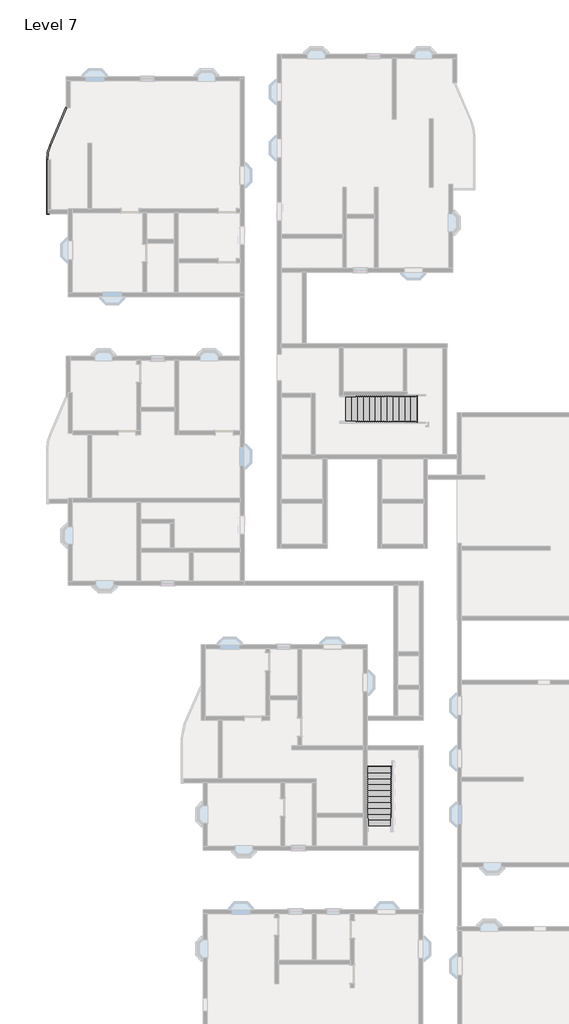
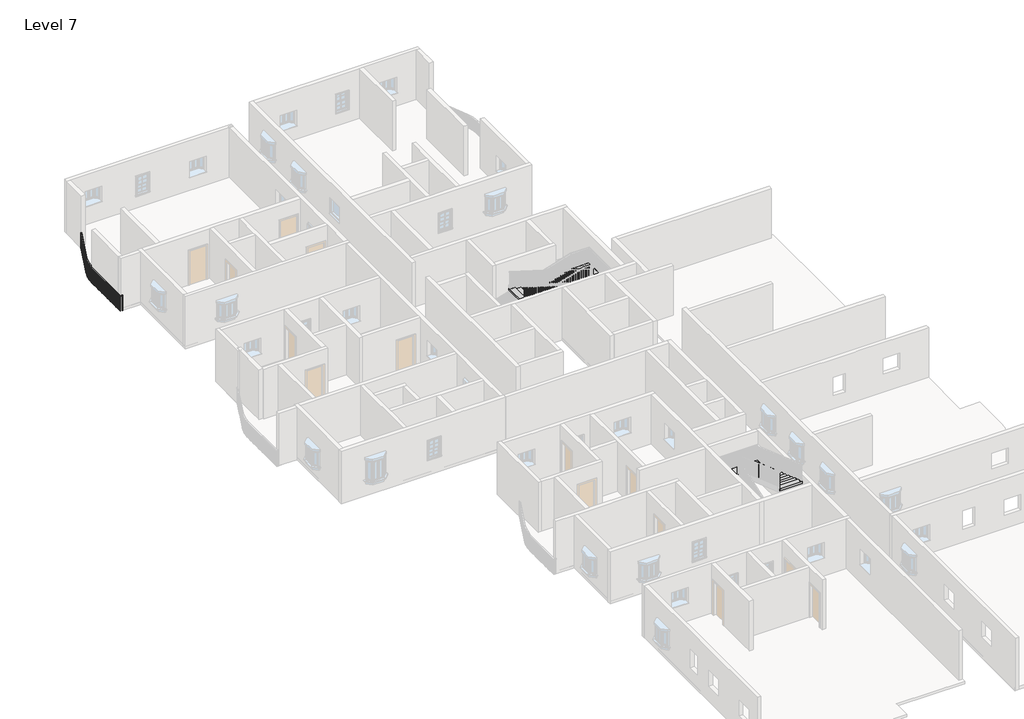
# One storey, part 12 of 14: 2 stair flights, 1 railing.
"""IFC4 building model written with IfcOpenShell, lengths in millimetres."""

from ifc_helpers import new_model, si_unit, frame, origin, place, context, project, spatial, polyline, circle_curve, outline, extrude, transform, mapped, element, save
from ifc_brep_helpers import plane_surface, cylinder_surface, revolved_surface, advanced_brep
from components import stair_flight_8b440c70, stair_flight_8f1750f9

model = new_model("IFC4")

# Units and contexts
model_context = context("Model", 3, world=origin())
ifc_project = project(units=[si_unit("LENGTHUNIT", "METRE", prefix="MILLI")], contexts=[model_context])

# Site, building, storey
site = spatial("IfcSite", under=ifc_project)
building = spatial("IfcBuilding", under=site)
storey = spatial("IfcBuildingStorey", under=building, Name="Level 7", Elevation=18288.0)

# Railing
placement = place(None, origin())
element("IfcRailing", 1, ObjectType="Handrail - Rectangular", at=placement, inside=storey, context=model_context, shape_type="SolidModel", body=[
    advanced_brep(
    [(-19327.739878, 27355.8257339, 19202.4), (-19327.739878, 27355.8257339, 19151.6), (-19374.4383922, 27375.822953, 19151.6), (-19374.4383922, 27375.822953, 19202.4), (-20162.483418, 25406.4905323, 19202.4), (-20162.483418, 25406.4905323, 19151.6), (-20209.1819322, 25426.4877514, 19151.6), (-20209.1819322, 25426.4877514, 19202.4), (-20316.2891351, 24656.5948172, 19151.6), (-20316.2891351, 24656.5948172, 19202.4), (-20367.0891351, 24656.5948172, 19151.6), (-20367.0891351, 24656.5948172, 19202.4), (-20316.2891351, 21915.0583494, 19202.4), (-20316.2891351, 21915.0583494, 19151.6), (-20367.0891351, 21864.2583494, 19151.6), (-20367.0891351, 21864.2583494, 19202.4), (-20240.0891351, 21915.0583494, 19202.4), (-20240.0891351, 21864.2583494, 19202.4), (-20240.0891351, 21864.2583494, 19151.6), (-20240.0891351, 21915.0583494, 19151.6)],
    [
        (0, 1),
        (1, 2),
        (2, 3),
        (3, 0),
        (0, 4),
        (4, 5),
        (5, 1),
        (5, 6),
        (6, 2),
        (6, 7),
        (7, 3),
        (7, 4),
        (8, 5, circle_curve(frame((-18411.2891351, 24656.5948172, 19151.6), z_axis=(0.0, 0.0, -1.0), x_axis=(-0.9192620907623792, 0.3936460446736121, 0.0)), 1905.0)),
        (4, 9, circle_curve(frame((-18411.2891351, 24656.5948172, 19202.4), z_axis=(0.0, 0.0, 1.0), x_axis=(-0.9192620907623792, 0.3936460446736121, 0.0)), 1905.0)),
        (9, 8),
        (10, 6, circle_curve(frame((-18411.2891351, 24656.5948172, 19151.6), z_axis=(0.0, 0.0, -1.0), x_axis=(-0.9192620907623792, 0.3936460446736121, 0.0)), 1955.8)),
        (8, 10),
        (11, 7, circle_curve(frame((-18411.2891351, 24656.5948172, 19202.4), z_axis=(0.0, 0.0, -1.0), x_axis=(-0.9192620907623792, 0.3936460446736121, 0.0)), 1955.8)),
        (10, 11),
        (11, 9),
        (9, 12),
        (12, 13),
        (13, 8),
        (13, 14),
        (14, 10),
        (14, 15),
        (15, 11),
        (15, 12),
        (16, 17),
        (17, 18),
        (18, 19),
        (19, 16),
        (12, 16),
        (19, 13),
        (18, 14),
        (17, 15),
    ],
    [
        plane_surface(frame((-19351.0891351, 27365.8243434, 19202.4), z_axis=(0.3936460446736102, 0.91926209076238, 0.0), x_axis=(0.91926209076238, -0.3936460446736102, 0.0))),
        plane_surface(frame((-19327.739878, 27355.8257339, 19202.4), z_axis=(0.91926209076238, -0.3936460446736102, 0.0), x_axis=(-0.3936460446736102, -0.91926209076238, 0.0))),
        plane_surface(frame((-19327.739878, 27355.8257339, 19151.6), z_axis=(0.0, 0.0, -1.0), x_axis=(-0.3936460446736102, -0.91926209076238, 0.0))),
        plane_surface(frame((-19374.4383922, 27375.822953, 19151.6), z_axis=(-0.91926209076238, 0.3936460446736102, 0.0), x_axis=(-0.3936460446736102, -0.91926209076238, 0.0))),
        plane_surface(frame((-19374.4383922, 27375.822953, 19202.4), z_axis=(0.0, 0.0, 1.0), x_axis=(-0.3936460446736102, -0.91926209076238, 0.0))),
        revolved_surface(polyline([(-20162.48341800233, 25406.49053230323, 19202.4), (-20162.48341800233, 25406.49053230323, 19151.6)]), (-18411.2891351, 24656.5948172, 19202.4), (0.0, 0.0, 1.0)),
        plane_surface(frame((-18411.2891351, 24656.5948172, 19151.6), z_axis=(0.0, 0.0, -1.0), x_axis=(-0.9192620907623792, 0.3936460446736121, 0.0))),
        cylinder_surface(frame((-18411.2891351, 24656.5948172, 19202.4), z_axis=(0.0, 0.0, 1.0), x_axis=(-0.9192620907623792, 0.3936460446736121, 0.0)), 1955.8),
        plane_surface(frame((-18411.2891351, 24656.5948172, 19202.4), z_axis=(0.0, 0.0, 1.0), x_axis=(-0.9192620907623792, 0.3936460446736121, 0.0))),
        plane_surface(frame((-20316.2891351, 24656.5948172, 19202.4), z_axis=(1.0, 0.0, 0.0), x_axis=(0.0, -1.0, 0.0))),
        plane_surface(frame((-20316.2891351, 24656.5948172, 19151.6), z_axis=(0.0, 0.0, -1.0), x_axis=(0.0, -1.0, 0.0))),
        plane_surface(frame((-20367.0891351, 24656.5948172, 19151.6), z_axis=(-1.0, 0.0, 0.0), x_axis=(0.0, -1.0, 0.0))),
        plane_surface(frame((-20367.0891351, 24656.5948172, 19202.4), z_axis=(0.0, 0.0, 1.0), x_axis=(0.0, -1.0, 0.0))),
        plane_surface(frame((-20240.0891351, 21889.6583494, 19202.4), z_axis=(1.0, 0.0, 0.0), x_axis=(0.0, 1.0, 0.0))),
        plane_surface(frame((-20316.2891351, 21915.0583494, 19202.4), z_axis=(0.0, 1.0, 0.0), x_axis=(1.0, 0.0, 0.0))),
        plane_surface(frame((-20316.2891351, 21915.0583494, 19151.6), z_axis=(0.0, 0.0, -1.0), x_axis=(1.0, 0.0, 0.0))),
        plane_surface(frame((-20367.0891351, 21864.2583494, 19151.6), z_axis=(0.0, -1.0, 0.0), x_axis=(1.0, 0.0, 0.0))),
        plane_surface(frame((-20367.0891351, 21864.2583494, 19202.4), z_axis=(0.0, 0.0, 1.0), x_axis=(1.0, 0.0, 0.0))),
    ],
    [
        (0, [[1, 2, 3, 4]]),
        (1, [[-1, 5, 6, 7]]),
        (2, [[-2, -7, 8, 9]]),
        (3, [[-3, -9, 10, 11]]),
        (4, [[-4, -11, 12, -5]]),
        (5, [[13, -6, 14, 15]]),
        (6, [[16, -8, -13, 17]]),
        (7, [[18, -10, -16, 19]]),
        (8, [[-14, -12, -18, 20]]),
        (9, [[-15, 21, 22, 23]]),
        (10, [[-17, -23, 24, 25]]),
        (11, [[-19, -25, 26, 27]]),
        (12, [[-20, -27, 28, -21]]),
        (13, [[29, 30, 31, 32]]),
        (14, [[-22, 33, -32, 34]]),
        (15, [[-24, -34, -31, 35]]),
        (16, [[-26, -35, -30, 36]]),
        (17, [[-28, -36, -29, -33]]),
    ],
),
    extrude(outline(polyline([(-20351.2141351, 21922.9198172), (-20332.1641351, 21922.9198172), (-20332.1641351, 21903.8698172), (-20351.2141351, 21903.8698172), (-20351.2141351, 21922.9198172)])), frame((0.0, 0.0, 18288.0), z_axis=(0.0, 0.0, 1.0), x_axis=(1.0, 0.0, 0.0)), (0.0, 0.0, 1.0), 863.6),
    extrude(outline(polyline([(-20351.2141351, 22024.5198172), (-20332.1641351, 22024.5198172), (-20332.1641351, 22005.4698172), (-20351.2141351, 22005.4698172), (-20351.2141351, 22024.5198172)])), frame((0.0, 0.0, 18288.0), z_axis=(0.0, 0.0, 1.0), x_axis=(1.0, 0.0, 0.0)), (0.0, 0.0, 1.0), 863.6),
    extrude(outline(polyline([(-20351.2141351, 22126.1198172), (-20332.1641351, 22126.1198172), (-20332.1641351, 22107.0698172), (-20351.2141351, 22107.0698172), (-20351.2141351, 22126.1198172)])), frame((0.0, 0.0, 18288.0), z_axis=(0.0, 0.0, 1.0), x_axis=(1.0, 0.0, 0.0)), (0.0, 0.0, 1.0), 863.6),
    extrude(outline(polyline([(-20351.2141351, 22227.7198172), (-20332.1641351, 22227.7198172), (-20332.1641351, 22208.6698172), (-20351.2141351, 22208.6698172), (-20351.2141351, 22227.7198172)])), frame((0.0, 0.0, 18288.0), z_axis=(0.0, 0.0, 1.0), x_axis=(1.0, 0.0, 0.0)), (0.0, 0.0, 1.0), 863.6),
    extrude(outline(polyline([(-20351.2141351, 22329.3198172), (-20332.1641351, 22329.3198172), (-20332.1641351, 22310.2698172), (-20351.2141351, 22310.2698172), (-20351.2141351, 22329.3198172)])), frame((0.0, 0.0, 18288.0), z_axis=(0.0, 0.0, 1.0), x_axis=(1.0, 0.0, 0.0)), (0.0, 0.0, 1.0), 863.6),
    extrude(outline(polyline([(-20351.2141351, 22430.9198172), (-20332.1641351, 22430.9198172), (-20332.1641351, 22411.8698172), (-20351.2141351, 22411.8698172), (-20351.2141351, 22430.9198172)])), frame((0.0, 0.0, 18288.0), z_axis=(0.0, 0.0, 1.0), x_axis=(1.0, 0.0, 0.0)), (0.0, 0.0, 1.0), 863.6),
    extrude(outline(polyline([(-20351.2141351, 22532.5198172), (-20332.1641351, 22532.5198172), (-20332.1641351, 22513.4698172), (-20351.2141351, 22513.4698172), (-20351.2141351, 22532.5198172)])), frame((0.0, 0.0, 18288.0), z_axis=(0.0, 0.0, 1.0), x_axis=(1.0, 0.0, 0.0)), (0.0, 0.0, 1.0), 863.6),
    extrude(outline(polyline([(-20351.2141351, 22634.1198172), (-20332.1641351, 22634.1198172), (-20332.1641351, 22615.0698172), (-20351.2141351, 22615.0698172), (-20351.2141351, 22634.1198172)])), frame((0.0, 0.0, 18288.0), z_axis=(0.0, 0.0, 1.0), x_axis=(1.0, 0.0, 0.0)), (0.0, 0.0, 1.0), 863.6),
    extrude(outline(polyline([(-20351.2141351, 22735.7198172), (-20332.1641351, 22735.7198172), (-20332.1641351, 22716.6698172), (-20351.2141351, 22716.6698172), (-20351.2141351, 22735.7198172)])), frame((0.0, 0.0, 18288.0), z_axis=(0.0, 0.0, 1.0), x_axis=(1.0, 0.0, 0.0)), (0.0, 0.0, 1.0), 863.6),
    extrude(outline(polyline([(-20351.2141351, 22837.3198172), (-20332.1641351, 22837.3198172), (-20332.1641351, 22818.2698172), (-20351.2141351, 22818.2698172), (-20351.2141351, 22837.3198172)])), frame((0.0, 0.0, 18288.0), z_axis=(0.0, 0.0, 1.0), x_axis=(1.0, 0.0, 0.0)), (0.0, 0.0, 1.0), 863.6),
    extrude(outline(polyline([(-20351.2141351, 22938.9198172), (-20332.1641351, 22938.9198172), (-20332.1641351, 22919.8698172), (-20351.2141351, 22919.8698172), (-20351.2141351, 22938.9198172)])), frame((0.0, 0.0, 18288.0), z_axis=(0.0, 0.0, 1.0), x_axis=(1.0, 0.0, 0.0)), (0.0, 0.0, 1.0), 863.6),
    extrude(outline(polyline([(-20351.2141351, 23040.5198172), (-20332.1641351, 23040.5198172), (-20332.1641351, 23021.4698172), (-20351.2141351, 23021.4698172), (-20351.2141351, 23040.5198172)])), frame((0.0, 0.0, 18288.0), z_axis=(0.0, 0.0, 1.0), x_axis=(1.0, 0.0, 0.0)), (0.0, 0.0, 1.0), 863.6),
    extrude(outline(polyline([(-20351.2141351, 23142.1198172), (-20332.1641351, 23142.1198172), (-20332.1641351, 23123.0698172), (-20351.2141351, 23123.0698172), (-20351.2141351, 23142.1198172)])), frame((0.0, 0.0, 18288.0), z_axis=(0.0, 0.0, 1.0), x_axis=(1.0, 0.0, 0.0)), (0.0, 0.0, 1.0), 863.6),
    extrude(outline(polyline([(-20351.2141351, 23243.7198172), (-20332.1641351, 23243.7198172), (-20332.1641351, 23224.6698172), (-20351.2141351, 23224.6698172), (-20351.2141351, 23243.7198172)])), frame((0.0, 0.0, 18288.0), z_axis=(0.0, 0.0, 1.0), x_axis=(1.0, 0.0, 0.0)), (0.0, 0.0, 1.0), 863.6),
    extrude(outline(polyline([(-20351.2141351, 23345.3198172), (-20332.1641351, 23345.3198172), (-20332.1641351, 23326.2698172), (-20351.2141351, 23326.2698172), (-20351.2141351, 23345.3198172)])), frame((0.0, 0.0, 18288.0), z_axis=(0.0, 0.0, 1.0), x_axis=(1.0, 0.0, 0.0)), (0.0, 0.0, 1.0), 863.6),
    extrude(outline(polyline([(-20351.2141351, 23446.9198172), (-20332.1641351, 23446.9198172), (-20332.1641351, 23427.8698172), (-20351.2141351, 23427.8698172), (-20351.2141351, 23446.9198172)])), frame((0.0, 0.0, 18288.0), z_axis=(0.0, 0.0, 1.0), x_axis=(1.0, 0.0, 0.0)), (0.0, 0.0, 1.0), 863.6),
    extrude(outline(polyline([(-20351.2141351, 23548.5198172), (-20332.1641351, 23548.5198172), (-20332.1641351, 23529.4698172), (-20351.2141351, 23529.4698172), (-20351.2141351, 23548.5198172)])), frame((0.0, 0.0, 18288.0), z_axis=(0.0, 0.0, 1.0), x_axis=(1.0, 0.0, 0.0)), (0.0, 0.0, 1.0), 863.6),
    extrude(outline(polyline([(-20351.2141351, 23650.1198172), (-20332.1641351, 23650.1198172), (-20332.1641351, 23631.0698172), (-20351.2141351, 23631.0698172), (-20351.2141351, 23650.1198172)])), frame((0.0, 0.0, 18288.0), z_axis=(0.0, 0.0, 1.0), x_axis=(1.0, 0.0, 0.0)), (0.0, 0.0, 1.0), 863.6),
    extrude(outline(polyline([(-20351.2141351, 23751.7198172), (-20332.1641351, 23751.7198172), (-20332.1641351, 23732.6698172), (-20351.2141351, 23732.6698172), (-20351.2141351, 23751.7198172)])), frame((0.0, 0.0, 18288.0), z_axis=(0.0, 0.0, 1.0), x_axis=(1.0, 0.0, 0.0)), (0.0, 0.0, 1.0), 863.6),
    extrude(outline(polyline([(-20351.2141351, 23853.3198172), (-20332.1641351, 23853.3198172), (-20332.1641351, 23834.2698172), (-20351.2141351, 23834.2698172), (-20351.2141351, 23853.3198172)])), frame((0.0, 0.0, 18288.0), z_axis=(0.0, 0.0, 1.0), x_axis=(1.0, 0.0, 0.0)), (0.0, 0.0, 1.0), 863.6),
    extrude(outline(polyline([(-20351.2141351, 23954.9198172), (-20332.1641351, 23954.9198172), (-20332.1641351, 23935.8698172), (-20351.2141351, 23935.8698172), (-20351.2141351, 23954.9198172)])), frame((0.0, 0.0, 18288.0), z_axis=(0.0, 0.0, 1.0), x_axis=(1.0, 0.0, 0.0)), (0.0, 0.0, 1.0), 863.6),
    extrude(outline(polyline([(-20351.2141351, 24056.5198172), (-20332.1641351, 24056.5198172), (-20332.1641351, 24037.4698172), (-20351.2141351, 24037.4698172), (-20351.2141351, 24056.5198172)])), frame((0.0, 0.0, 18288.0), z_axis=(0.0, 0.0, 1.0), x_axis=(1.0, 0.0, 0.0)), (0.0, 0.0, 1.0), 863.6),
    extrude(outline(polyline([(-20351.2141351, 24158.1198172), (-20332.1641351, 24158.1198172), (-20332.1641351, 24139.0698172), (-20351.2141351, 24139.0698172), (-20351.2141351, 24158.1198172)])), frame((0.0, 0.0, 18288.0), z_axis=(0.0, 0.0, 1.0), x_axis=(1.0, 0.0, 0.0)), (0.0, 0.0, 1.0), 863.6),
    extrude(outline(polyline([(-20351.2141351, 24259.7198172), (-20332.1641351, 24259.7198172), (-20332.1641351, 24240.6698172), (-20351.2141351, 24240.6698172), (-20351.2141351, 24259.7198172)])), frame((0.0, 0.0, 18288.0), z_axis=(0.0, 0.0, 1.0), x_axis=(1.0, 0.0, 0.0)), (0.0, 0.0, 1.0), 863.6),
    extrude(outline(polyline([(-20351.2141351, 24361.3198172), (-20332.1641351, 24361.3198172), (-20332.1641351, 24342.2698172), (-20351.2141351, 24342.2698172), (-20351.2141351, 24361.3198172)])), frame((0.0, 0.0, 18288.0), z_axis=(0.0, 0.0, 1.0), x_axis=(1.0, 0.0, 0.0)), (0.0, 0.0, 1.0), 863.6),
    extrude(outline(polyline([(-20351.2141351, 24462.9198172), (-20332.1641351, 24462.9198172), (-20332.1641351, 24443.8698172), (-20351.2141351, 24443.8698172), (-20351.2141351, 24462.9198172)])), frame((0.0, 0.0, 18288.0), z_axis=(0.0, 0.0, 1.0), x_axis=(1.0, 0.0, 0.0)), (0.0, 0.0, 1.0), 863.6),
    extrude(outline(polyline([(-20351.2141351, 24564.5198172), (-20332.1641351, 24564.5198172), (-20332.1641351, 24545.4698172), (-20351.2141351, 24545.4698172), (-20351.2141351, 24564.5198172)])), frame((0.0, 0.0, 18288.0), z_axis=(0.0, 0.0, 1.0), x_axis=(1.0, 0.0, 0.0)), (0.0, 0.0, 1.0), 863.6),
    extrude(outline(polyline([(-20349.6005818, 24736.2720848), (-20330.5630441, 24735.5831307), (-20331.2519982, 24716.545593), (-20350.289536, 24717.2345471), (-20349.6005818, 24736.2720848)])), frame((0.0, 0.0, 18288.0), z_axis=(0.0, 0.0, 1.0), x_axis=(1.0, 0.0, 0.0)), (0.0, 0.0, 1.0), 863.6),
    extrude(outline(polyline([(-20342.724955, 24838.1310534), (-20323.750023, 24836.4415402), (-20325.4395363, 24817.4666081), (-20344.4144683, 24819.1561214), (-20342.724955, 24838.1310534)])), frame((0.0, 0.0, 18288.0), z_axis=(0.0, 0.0, 1.0), x_axis=(1.0, 0.0, 0.0)), (0.0, 0.0, 1.0), 863.6),
    extrude(outline(polyline([(-20330.5003254, 24939.4872677), (-20311.6405491, 24936.8018743), (-20314.3259425, 24917.942098), (-20333.1857188, 24920.6274914), (-20330.5003254, 24939.4872677)])), frame((0.0, 0.0, 18288.0), z_axis=(0.0, 0.0, 1.0), x_axis=(1.0, 0.0, 0.0)), (0.0, 0.0, 1.0), 863.6),
    extrude(outline(polyline([(-20312.9605484, 25040.0600272), (-20294.2681589, 25036.3861907), (-20297.9419954, 25017.6938012), (-20316.6343849, 25021.3676377), (-20312.9605484, 25040.0600272)])), frame((0.0, 0.0, 18288.0), z_axis=(0.0, 0.0, 1.0), x_axis=(1.0, 0.0, 0.0)), (0.0, 0.0, 1.0), 863.6),
    extrude(outline(polyline([(-20290.1541995, 25139.5708014), (-20271.6809643, 25134.9186963), (-20276.3330693, 25116.4454611), (-20294.8063045, 25121.0975662), (-20290.1541995, 25139.5708014)])), frame((0.0, 0.0, 18288.0), z_axis=(0.0, 0.0, 1.0), x_axis=(1.0, 0.0, 0.0)), (0.0, 0.0, 1.0), 863.6),
    extrude(outline(polyline([(-20262.1444395, 25237.7440008), (-20243.9415192, 25232.1265109), (-20249.5590091, 25213.9235906), (-20267.7619294, 25219.5410805), (-20262.1444395, 25237.7440008)])), frame((0.0, 0.0, 18288.0), z_axis=(0.0, 0.0, 1.0), x_axis=(1.0, 0.0, 0.0)), (0.0, 0.0, 1.0), 863.6),
    extrude(outline(polyline([(-20229.0088399, 25334.3077402), (-20211.1266465, 25327.7404228), (-20217.693964, 25309.8582293), (-20235.5761574, 25316.4255468), (-20229.0088399, 25334.3077402)])), frame((0.0, 0.0, 18288.0), z_axis=(0.0, 0.0, 1.0), x_axis=(1.0, 0.0, 0.0)), (0.0, 0.0, 1.0), 863.6),
    extrude(outline(polyline([(-20155.9843907, 25510.389225), (-20138.4724479, 25502.8902678), (-20145.9714051, 25485.378325), (-20163.4833479, 25492.8772822), (-20155.9843907, 25510.389225)])), frame((0.0, 0.0, 18288.0), z_axis=(0.0, 0.0, 1.0), x_axis=(1.0, 0.0, 0.0)), (0.0, 0.0, 1.0), 863.6),
    extrude(outline(polyline([(-20115.9899526, 25603.7862534), (-20098.4780098, 25596.2872963), (-20105.9769669, 25578.7753534), (-20123.4889098, 25586.2743106), (-20115.9899526, 25603.7862534)])), frame((0.0, 0.0, 18288.0), z_axis=(0.0, 0.0, 1.0), x_axis=(1.0, 0.0, 0.0)), (0.0, 0.0, 1.0), 863.6),
    extrude(outline(polyline([(-20075.9955145, 25697.1832818), (-20058.4835716, 25689.6843247), (-20065.9825288, 25672.1723818), (-20083.4944716, 25679.671339), (-20075.9955145, 25697.1832818)])), frame((0.0, 0.0, 18288.0), z_axis=(0.0, 0.0, 1.0), x_axis=(1.0, 0.0, 0.0)), (0.0, 0.0, 1.0), 863.6),
    extrude(outline(polyline([(-20036.0010763, 25790.5803103), (-20018.4891335, 25783.0813531), (-20025.9880906, 25765.5694103), (-20043.5000335, 25773.0683674), (-20036.0010763, 25790.5803103)])), frame((0.0, 0.0, 18288.0), z_axis=(0.0, 0.0, 1.0), x_axis=(1.0, 0.0, 0.0)), (0.0, 0.0, 1.0), 863.6),
    extrude(outline(polyline([(-19996.0066382, 25883.9773387), (-19978.4946954, 25876.4783815), (-19985.9936525, 25858.9664387), (-20003.5055953, 25866.4653958), (-19996.0066382, 25883.9773387)])), frame((0.0, 0.0, 18288.0), z_axis=(0.0, 0.0, 1.0), x_axis=(1.0, 0.0, 0.0)), (0.0, 0.0, 1.0), 863.6),
    extrude(outline(polyline([(-19956.0122, 25977.3743671), (-19938.5002572, 25969.8754099), (-19945.9992144, 25952.3634671), (-19963.5111572, 25959.8624243), (-19956.0122, 25977.3743671)])), frame((0.0, 0.0, 18288.0), z_axis=(0.0, 0.0, 1.0), x_axis=(1.0, 0.0, 0.0)), (0.0, 0.0, 1.0), 863.6),
    extrude(outline(polyline([(-19916.0177619, 26070.7713955), (-19898.5058191, 26063.2724384), (-19906.0047762, 26045.7604955), (-19923.5167191, 26053.2594527), (-19916.0177619, 26070.7713955)])), frame((0.0, 0.0, 18288.0), z_axis=(0.0, 0.0, 1.0), x_axis=(1.0, 0.0, 0.0)), (0.0, 0.0, 1.0), 863.6),
    extrude(outline(polyline([(-19876.0233238, 26164.1684239), (-19858.5113809, 26156.6694668), (-19866.0103381, 26139.157524), (-19883.5222809, 26146.6564811), (-19876.0233238, 26164.1684239)])), frame((0.0, 0.0, 18288.0), z_axis=(0.0, 0.0, 1.0), x_axis=(1.0, 0.0, 0.0)), (0.0, 0.0, 1.0), 863.6),
    extrude(outline(polyline([(-19836.0288856, 26257.5654524), (-19818.5169428, 26250.0664952), (-19826.0159, 26232.5545524), (-19843.5278428, 26240.0535095), (-19836.0288856, 26257.5654524)])), frame((0.0, 0.0, 18288.0), z_axis=(0.0, 0.0, 1.0), x_axis=(1.0, 0.0, 0.0)), (0.0, 0.0, 1.0), 863.6),
    extrude(outline(polyline([(-19796.0344475, 26350.9624808), (-19778.5225047, 26343.4635236), (-19786.0214618, 26325.9515808), (-19803.5334046, 26333.450538), (-19796.0344475, 26350.9624808)])), frame((0.0, 0.0, 18288.0), z_axis=(0.0, 0.0, 1.0), x_axis=(1.0, 0.0, 0.0)), (0.0, 0.0, 1.0), 863.6),
    extrude(outline(polyline([(-19756.0400094, 26444.3595092), (-19738.5280665, 26436.860552), (-19746.0270237, 26419.3486092), (-19763.5389665, 26426.8475664), (-19756.0400094, 26444.3595092)])), frame((0.0, 0.0, 18288.0), z_axis=(0.0, 0.0, 1.0), x_axis=(1.0, 0.0, 0.0)), (0.0, 0.0, 1.0), 863.6),
    extrude(outline(polyline([(-19716.0455712, 26537.7565376), (-19698.5336284, 26530.2575805), (-19706.0325855, 26512.7456376), (-19723.5445284, 26520.2445948), (-19716.0455712, 26537.7565376)])), frame((0.0, 0.0, 18288.0), z_axis=(0.0, 0.0, 1.0), x_axis=(1.0, 0.0, 0.0)), (0.0, 0.0, 1.0), 863.6),
    extrude(outline(polyline([(-19676.0511331, 26631.153566), (-19658.5391902, 26623.6546089), (-19666.0381474, 26606.1426661), (-19683.5500902, 26613.6416232), (-19676.0511331, 26631.153566)])), frame((0.0, 0.0, 18288.0), z_axis=(0.0, 0.0, 1.0), x_axis=(1.0, 0.0, 0.0)), (0.0, 0.0, 1.0), 863.6),
    extrude(outline(polyline([(-19636.0566949, 26724.5505945), (-19618.5447521, 26717.0516373), (-19626.0437093, 26699.5396945), (-19643.5556521, 26707.0386516), (-19636.0566949, 26724.5505945)])), frame((0.0, 0.0, 18288.0), z_axis=(0.0, 0.0, 1.0), x_axis=(1.0, 0.0, 0.0)), (0.0, 0.0, 1.0), 863.6),
    extrude(outline(polyline([(-19596.0622568, 26817.9476229), (-19578.550314, 26810.4486657), (-19586.0492711, 26792.9367229), (-19603.561214, 26800.4356801), (-19596.0622568, 26817.9476229)])), frame((0.0, 0.0, 18288.0), z_axis=(0.0, 0.0, 1.0), x_axis=(1.0, 0.0, 0.0)), (0.0, 0.0, 1.0), 863.6),
    extrude(outline(polyline([(-19556.0678187, 26911.3446513), (-19538.5558758, 26903.8456942), (-19546.054833, 26886.3337513), (-19563.5667758, 26893.8327085), (-19556.0678187, 26911.3446513)])), frame((0.0, 0.0, 18288.0), z_axis=(0.0, 0.0, 1.0), x_axis=(1.0, 0.0, 0.0)), (0.0, 0.0, 1.0), 863.6),
    extrude(outline(polyline([(-19516.0733805, 27004.7416797), (-19498.5614377, 26997.2427226), (-19506.0603948, 26979.7307797), (-19523.5723377, 26987.2297369), (-19516.0733805, 27004.7416797)])), frame((0.0, 0.0, 18288.0), z_axis=(0.0, 0.0, 1.0), x_axis=(1.0, 0.0, 0.0)), (0.0, 0.0, 1.0), 863.6),
    extrude(outline(polyline([(-19476.0789424, 27098.1387082), (-19458.5669996, 27090.639751), (-19466.0659567, 27073.1278082), (-19483.5778995, 27080.6267653), (-19476.0789424, 27098.1387082)])), frame((0.0, 0.0, 18288.0), z_axis=(0.0, 0.0, 1.0), x_axis=(1.0, 0.0, 0.0)), (0.0, 0.0, 1.0), 863.6),
    extrude(outline(polyline([(-19436.0845042, 27191.5357366), (-19418.5725614, 27184.0367794), (-19426.0715186, 27166.5248366), (-19443.5834614, 27174.0237937), (-19436.0845042, 27191.5357366)])), frame((0.0, 0.0, 18288.0), z_axis=(0.0, 0.0, 1.0), x_axis=(1.0, 0.0, 0.0)), (0.0, 0.0, 1.0), 863.6),
    extrude(outline(polyline([(-19396.0900661, 27284.932765), (-19378.5781233, 27277.4338078), (-19386.0770804, 27259.921865), (-19403.5890233, 27267.4208222), (-19396.0900661, 27284.932765)])), frame((0.0, 0.0, 18288.0), z_axis=(0.0, 0.0, 1.0), x_axis=(1.0, 0.0, 0.0)), (0.0, 0.0, 1.0), 863.6),
    extrude(outline(polyline([(-20351.2141351, 21899.1833494), (-20332.1641351, 21899.1833494), (-20332.1641351, 21880.1333494), (-20351.2141351, 21880.1333494), (-20351.2141351, 21899.1833494)])), frame((0.0, 0.0, 18288.0), z_axis=(0.0, 0.0, 1.0), x_axis=(1.0, 0.0, 0.0)), (0.0, 0.0, 1.0), 863.6),
    extrude(outline(polyline([(-20351.2141351, 24666.1198172), (-20332.1641351, 24666.1198172), (-20332.1641351, 24647.0698172), (-20351.2141351, 24647.0698172), (-20351.2141351, 24666.1198172)])), frame((0.0, 0.0, 18288.0), z_axis=(0.0, 0.0, 1.0), x_axis=(1.0, 0.0, 0.0)), (0.0, 0.0, 1.0), 863.6),
    extrude(outline(polyline([(-20190.839168, 25428.9945919), (-20173.3272251, 25421.4956347), (-20180.8261823, 25403.9836919), (-20198.3381251, 25411.482649), (-20190.839168, 25428.9945919)])), frame((0.0, 0.0, 18288.0), z_axis=(0.0, 0.0, 1.0), x_axis=(1.0, 0.0, 0.0)), (0.0, 0.0, 1.0), 863.6),
    extrude(outline(polyline([(-20259.1391351, 21880.1333494), (-20259.1391351, 21899.1833494), (-20240.0891351, 21899.1833494), (-20240.0891351, 21880.1333494), (-20259.1391351, 21880.1333494)])), frame((0.0, 0.0, 18288.0), z_axis=(0.0, 0.0, 1.0), x_axis=(1.0, 0.0, 0.0)), (0.0, 0.0, 1.0), 863.6),
    extrude(outline(polyline([(-19359.8451065, 27369.573822), (-19342.3331637, 27362.0748648), (-19349.8321209, 27344.562922), (-19367.3440637, 27352.0618792), (-19359.8451065, 27369.573822)])), frame((0.0, 0.0, 18288.0), z_axis=(0.0, 0.0, 1.0), x_axis=(1.0, 0.0, 0.0)), (0.0, 0.0, 1.0), 863.6),
])

# Stair flights
stair_flight_shape = stair_flight_8b440c70(model_context)
element("IfcStairFlight", 2, ObjectType="2\" Tread 1\" Nosing 1/4\" Riser", at=placement, inside=storey, context=model_context, shape_type="MappedRepresentation", body=[
    mapped(stair_flight_shape, transform((0.0, 0.0, 0.0), x_axis=(1.0, 0.0, 0.0), y_axis=(0.0, 1.0, 0.0), z_axis=(0.0, 0.0, 1.0))),
])
stair_flight_2_shape = stair_flight_8f1750f9(model_context)
element("IfcStairFlight", 3, ObjectType="2\" Tread 1\" Nosing 1/4\" Riser", at=placement, inside=storey, context=model_context, shape_type="MappedRepresentation", body=[
    mapped(stair_flight_2_shape, transform((0.0, 0.0, 0.0), x_axis=(1.0, 0.0, 0.0), y_axis=(0.0, 1.0, 0.0), z_axis=(0.0, 0.0, 1.0))),
])

save(model, "model.ifc")

# Revit data of these elements
# Type "Handrail - Rectangular"
#   Assembly Code = "C2010400"
#   built-in parameter 1008612 = 0.0416667 (stored number, unit not read)
#   built-in parameter 1008611 = 0.0416667 (stored number, unit not read)
#   built-in parameter 1008609 = 0.333333 (stored number, unit not read)
#   built-in parameter 1008604 = 0.166667 (stored number, unit not read)
#   built-in parameter 1008603 = 0.166667 (stored number, unit not read)
#   Railing Height = 3' - 0"
#   built-in parameter 1008630 = 2
#   built-in parameter 1008610 = 2
#   built-in parameter 1008618 = Baluster - Square : 3/4"
# Element 1 (IfcRailing, "Handrail - Rectangular")
#   Phase Created = New Construction
# Elements 2, 3 (IfcStairFlight, "2\" Tread 1\" Nosing 1/4\" Riser")
#   Phase Created = New Construction
